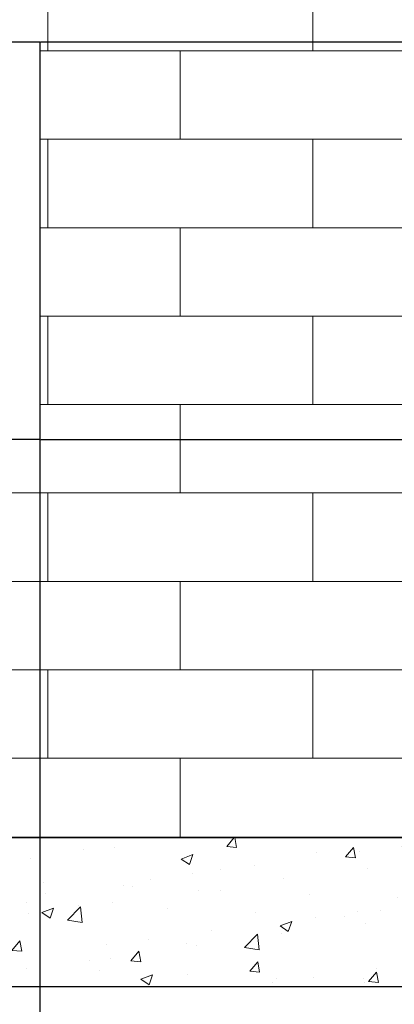
# Model space of a CAD drawing. Units: inches. Extents: x 37 to 824, y -700 to 234.
# Tile 10 of 77: x 253 to 298, y -606 to -487. Entities that reach past the tile are written whole.
import ezdxf

# ---------------------------------------------------------------- set-up
doc = ezdxf.new("R2010")
doc.units = ezdxf.units.IN
doc.header["$MEASUREMENT"] = 0
for name, color, linetype, lineweight in [('A-ANNO-DIMS', 2, 'Continuous', 18), ('A-ELEV', 3, 'Continuous', 25), ('A-ELEV-PATT', 8, 'Continuous', 13)]:
    doc.layers.add(name, color=color, linetype=linetype, lineweight=lineweight)
doc.styles.get("Standard").update_dxf_attribs({"font": 'arial.ttf'})
doc.dimstyles.get("Standard").update_dxf_attribs({"dimtxt": 0.18, "dimasz": 0.18, "dimexe": 0.18, "dimexo": 0.0625, "dimgap": 0.09, "dimtad": 0, "dimtih": 1, "dimtoh": 1, "dimdec": 1, "dimzin": 0, "dimdsep": 46, "dimlunit": 4, "dimtxsty": 'Standard', "dimcen": 0.09, "dimadec": 0, "dimazin": 0, "dimtfac": 1, "dimtdec": 1, "dimtofl": 0, "dimtmove": 0, "dimatfit": 3, "dimfxl": 1, "dimtolj": 1, "dimtzin": 0, "dimarcsym": 0})

# ---------------------------------------------------------------- blocks, each defined once
blk = doc.blocks.new('*D28')
at = {"layer": 'A-ANNO-DIMS', "color": 0, "lineweight": -2, "ltscale": 0.5, "transparency": 16777216}
for p, q in [((255.14, -537.63), (449.87, -537.63)), ((449.69, -543.63), (449.69, -558.54)), ((449.69, -579.63), (449.69, -564.72)), ((294.64, -585.63), (449.87, -585.63))]:
    blk.add_line(p, q, dxfattribs=at)
at = {"layer": 'A-ANNO-DIMS', "color": 0, "ltscale": 0.5, "transparency": 16777216}
for points in [[(448.69, -543.63), (450.69, -543.63), (449.69, -537.63)], [(448.69, -579.63), (450.69, -579.63), (449.69, -585.63)]]:
    blk.add_solid(points, dxfattribs=at)
at = {"layer": 'Defpoints', "color": 0, "ltscale": 0.5, "transparency": 16777216}
for p in [(255.08, -537.63), (294.58, -585.63), (449.69, -585.63)]:
    blk.add_point(p, dxfattribs=at)
at = {"layer": 'A-ANNO-DIMS', "color": 0, "ltscale": 0.5, "transparency": 16777216, "insert": (449.69, -561.63), "char_height": 6, "attachment_point": 5}
blk.add_mtext("\\A1;4'", dxfattribs=at)
blk = doc.blocks.new('*D31')
at = {"layer": 'A-ANNO-DIMS', "color": 0, "lineweight": -2, "ltscale": 0.5, "transparency": 16777216}
for p, q in [((255.14, -489.63), (449.77, -489.63)), ((449.59, -495.63), (449.59, -510.54)), ((449.59, -531.63), (449.59, -516.72)), ((255.14, -537.63), (449.77, -537.63))]:
    blk.add_line(p, q, dxfattribs=at)
at = {"layer": 'A-ANNO-DIMS', "color": 0, "ltscale": 0.5, "transparency": 16777216}
for points in [[(448.59, -495.63), (450.59, -495.63), (449.59, -489.63)], [(448.59, -531.63), (450.59, -531.63), (449.59, -537.63)]]:
    blk.add_solid(points, dxfattribs=at)
at = {"layer": 'Defpoints', "color": 0, "ltscale": 0.5, "transparency": 16777216}
for p in [(255.08, -489.63), (449.59, -489.63), (255.08, -537.63)]:
    blk.add_point(p, dxfattribs=at)
at = {"layer": 'A-ANNO-DIMS', "color": 0, "ltscale": 0.5, "transparency": 16777216, "insert": (449.59, -513.63), "char_height": 6, "attachment_point": 5}
blk.add_mtext("\\A1;4'", dxfattribs=at)
blk = doc.blocks.new('*D68')
at = {"layer": 'A-ANNO-DIMS', "color": 0, "lineweight": -2, "ltscale": 0.5, "transparency": 16777216}
for p, q in [((205.08, -537.69), (205.08, -699.59)), ((255.08, -537.69), (255.08, -699.59)), ((205.26, -699.41), (229.74, -699.41)), ((254.9, -699.41), (230.41, -699.41))]:
    blk.add_line(p, q, dxfattribs=at)
at = {"layer": 'A-ANNO-DIMS', "color": 0, "ltscale": 0.5, "transparency": 16777216}
for points in [[(205.26, -699.38), (205.26, -699.44), (205.08, -699.41)], [(254.9, -699.38), (254.9, -699.44), (255.08, -699.41)]]:
    blk.add_solid(points, dxfattribs=at)
at = {"layer": 'Defpoints', "color": 0, "ltscale": 0.5, "transparency": 16777216}
for p in [(205.08, -537.63), (255.08, -537.63), (255.08, -699.41)]:
    blk.add_point(p, dxfattribs=at)
at = {"layer": 'A-ANNO-DIMS', "color": 0, "ltscale": 0.5, "transparency": 16777216, "insert": (230.08, -699.41), "char_height": 0.18, "attachment_point": 5}
blk.add_mtext('\\A1;4\'-2"', dxfattribs=at)
blk = doc.blocks.new('*D69')
at = {"layer": 'A-ANNO-DIMS', "color": 0, "lineweight": -2, "ltscale": 0.5, "transparency": 16777216}
for p, q in [((255.08, -537.69), (255.08, -699.59)), ((299.08, -585.69), (299.08, -699.59)), ((255.26, -699.41), (276.75, -699.41)), ((298.9, -699.41), (277.41, -699.41))]:
    blk.add_line(p, q, dxfattribs=at)
at = {"layer": 'A-ANNO-DIMS', "color": 0, "ltscale": 0.5, "transparency": 16777216}
for points in [[(255.26, -699.38), (255.26, -699.44), (255.08, -699.41)], [(298.9, -699.38), (298.9, -699.44), (299.08, -699.41)]]:
    blk.add_solid(points, dxfattribs=at)
at = {"layer": 'Defpoints', "color": 0, "ltscale": 0.5, "transparency": 16777216}
for p in [(255.08, -537.63), (299.08, -585.63), (299.08, -699.41)]:
    blk.add_point(p, dxfattribs=at)
at = {"layer": 'A-ANNO-DIMS', "color": 0, "ltscale": 0.5, "transparency": 16777216, "insert": (277.08, -699.41), "char_height": 0.18, "attachment_point": 5}
blk.add_mtext('\\A1;3\'-8"', dxfattribs=at)

msp = doc.modelspace()

# ---------------------------------------------------------------- hatches: boundary and pattern name
at = {"layer": 'A-ELEV-PATT', "ltscale": 0.5}
h = msp.add_hatch(dxfattribs=at)
h.set_pattern_fill('AR-BRSTD', color=256, scale=4)
h.paths.add_polyline_path([(299.08, -489.63), (358.13, -489.63), (358.13, -585.63), (428.08, -585.63), (428.08, -465.63), (161.08, -465.63), (161.08, -585.63), (299.08, -585.63)])
h.paths.add_polyline_path([(205.08, -537.63), (205.08, -489.63), (255.08, -489.63), (255.08, -537.63)], flags=16)
h = msp.add_hatch(dxfattribs=at)
h.set_pattern_fill('AR-CONC', color=256, scale=2)
h.paths.add_polyline_path([(299.08, -585.63), (161.08, -585.63), (161.08, -603.63), (299.08, -603.63)])
h.paths.add_polyline_path([(428.08, -585.63), (358.13, -585.63), (358.13, -603.63), (428.08, -603.63)])

# ---------------------------------------------------------------- linework, layer by layer
at = {"layer": 'A-ELEV', "ltscale": 0.5}
for points in [[(161.08, -465.63), (428.08, -465.63), (428.08, -585.63), (161.08, -585.63)], [(205.08, -489.63), (255.08, -489.63), (255.08, -537.63), (205.08, -537.63)], [(161.08, -585.63), (428.08, -585.63), (428.08, -603.63), (161.08, -603.63)]]:
    msp.add_lwpolyline(points, close=True, dxfattribs=at)

# ---------------------------------------------------------------- dimensions: what is measured, and where the dimension line sits
at = {"layer": 'A-ANNO-DIMS', "ltscale": 0.5}
for base, p2, picture, middle in [((449.59, -489.63), (255.08, -489.63), '*D31', (449.59, -513.63)), ((449.69, -585.63), (294.58, -585.63), '*D28', (449.69, -561.63))]:
    dim = msp.add_linear_dim(base=base, p1=(255.08, -537.63), p2=p2, angle=90, dimstyle='Standard', override={"dimtxt": 6, "dimasz": 6, "dimclrd": 0, "dimclre": 0, "dimclrt": 0}, dxfattribs=at)
    dim.commit()
    dim.dimension.update_dxf_attribs({"geometry": picture, "text_midpoint": middle})
for base, p1, p2, picture, middle in [((255.08, -699.41), (205.08, -537.63), (255.08, -537.63), '*D68', (230.08, -699.41)), ((299.08, -699.41), (255.08, -537.63), (299.08, -585.63), '*D69', (277.08, -699.41))]:
    dim = msp.add_linear_dim(base=base, p1=p1, p2=p2, dimstyle='Standard', override={"dimdec": 1, "dimlfac": 1, "dimrnd": 0, "dimzin": 1, "dimdsep": 46, "dimlunit": 4, "dimfrac": 2}, dxfattribs=at)
    dim.commit()
    dim.dimension.update_dxf_attribs({"geometry": picture, "text_midpoint": middle})

doc.saveas('drawing.dxf')
